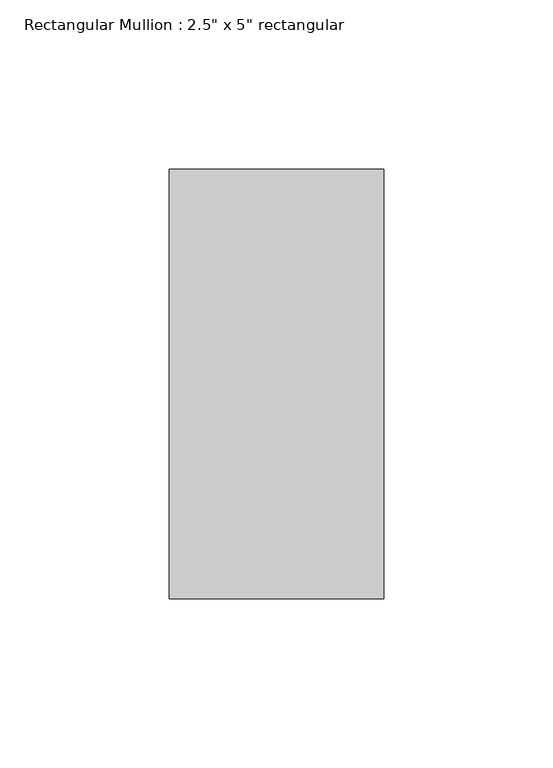
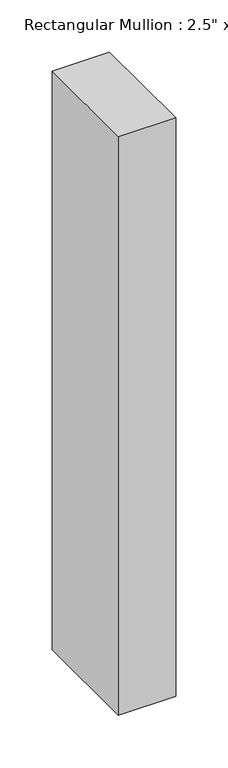
"""IFC4 building model written with IfcOpenShell, lengths in millimetres: member geometry."""

from ifc_helpers import new_model, si_unit, frame, origin, place, context, project, spatial, polyline, outline, extrude, source, transform, mapped, element, save


def member_baa20d8e(model_context):
    return source(origin(), model_context, "Body", "SweptSolid", [
        extrude(outline(polyline([(31.75, 63.5), (31.75, -63.5), (-31.75, -63.5), (-31.75, 63.5), (31.75, 63.5)])), frame((0.0, 0.0, -677.9496655), z_axis=(0.0, 0.0, 1.0), x_axis=(1.0, 0.0, 0.0)), (0.0, 0.0, 1.0), 677.9496655),
    ])


if __name__ == "__main__":
    model = new_model("IFC4")
    model_context = context("Model", 3, world=origin())
    ifc_project = project(units=[si_unit("LENGTHUNIT", "METRE", prefix="MILLI")], contexts=[model_context])
    site = spatial("IfcSite", under=ifc_project)
    building = spatial("IfcBuilding", under=site)
    placement = place(None, origin())
    member_shape = member_baa20d8e(model_context)
    element("IfcMember", 1, ObjectType="Rectangular Mullion : 2.5\" x 5\" rectangular", at=placement, inside=building, context=model_context, shape_type="MappedRepresentation", body=[
        mapped(member_shape, transform((0.0, 0.0, 0.0), x_axis=(1.0, 0.0, 0.0), y_axis=(0.0, 1.0, 0.0), z_axis=(0.0, 0.0, 1.0))),
    ])
    save(model, "model.ifc")

# Revit data of these elements
# Type "Rectangular Mullion : 2.5\" x 5\" rectangular"
#   built-in parameter 1007304 = 0.416667 (stored number, unit not read)
#   built-in parameter 1007301 = 0.104167 (stored number, unit not read)
#   built-in parameter 1007300 = 0.104167 (stored number, unit not read)
# Element 1 (IfcMember, "Rectangular Mullion : 2.5\" x 5\" rectangular")
#   Materials on its faces: "Aluminum"
# Materials
#   "Aluminum": class "Metal", colour RGB 247 247 247, transparency 0, Description = "Aluminum 6061", Cost = 0
